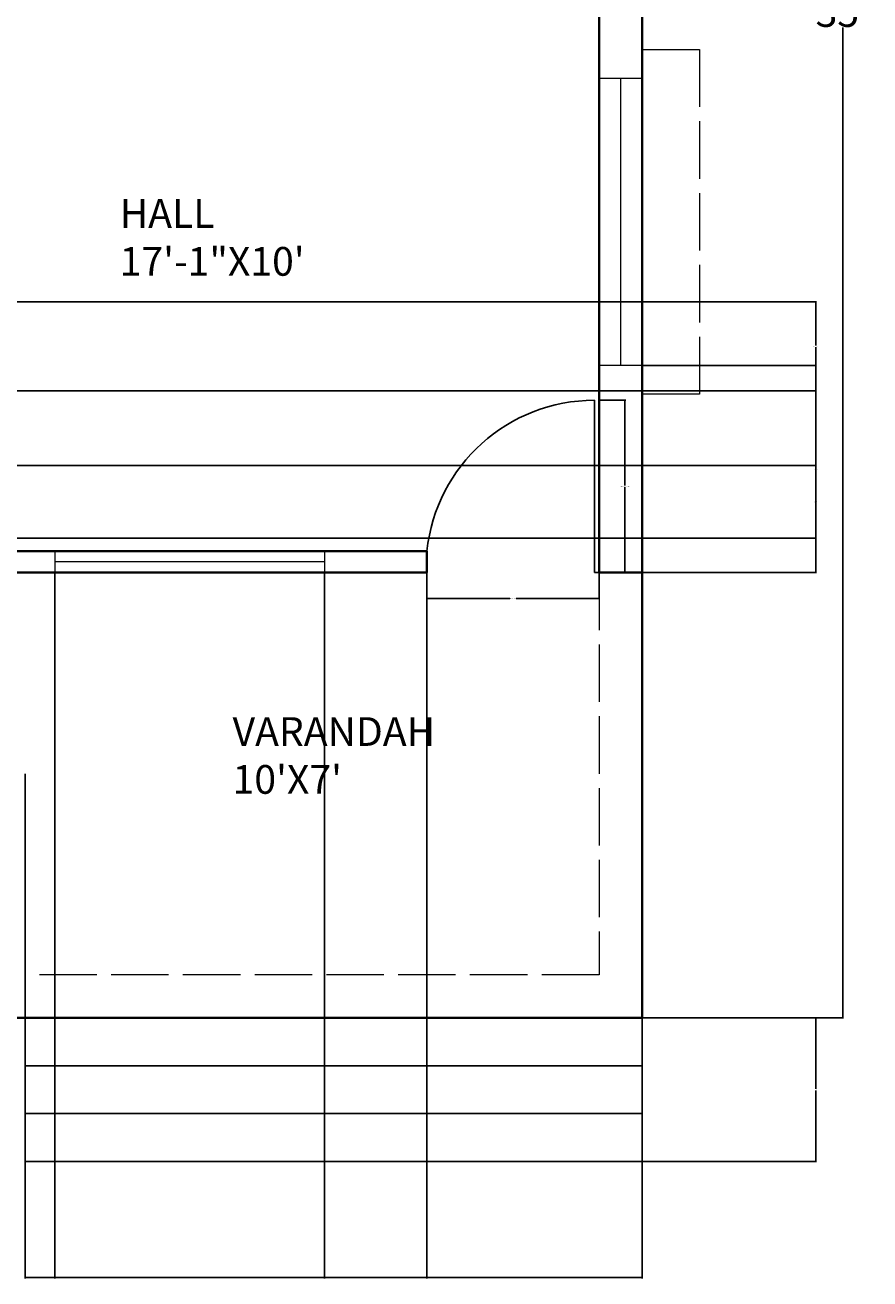
# Model space of a CAD drawing. Units: inches. Extents: x -22 to 362, y -469 to 42.
# Tile 3 of 6: x 186 to 362, y -469 to -207. Entities that reach past the tile are written whole.
import ezdxf

# ---------------------------------------------------------------- set-up
doc = ezdxf.new("R2010")
doc.units = ezdxf.units.IN
doc.header["$MEASUREMENT"] = 0
doc.linetypes.add('ACAD_ISO02W100', pattern=[15, 12, -3])
for name, color, linetype, lineweight in [('A-ANNO-DIMS', 2, 'Continuous', 18), ('A-AREA-IDEN', 7, 'Continuous', 25), ('A-DOOR', 3, 'Continuous', 25), ('A-FLOR-STRS', 7, 'Continuous', 25), ('A-GLAZ', 4, 'Continuous', 20), ('A-ROOF-OVHD', 8, 'ACAD_ISO02W100', 18), ('A-WALL', 7, 'Continuous', 40), ('A-WALL-OVHD', 7, 'ACAD_ISO02W100', 18)]:
    doc.layers.add(name, color=color, linetype=linetype, lineweight=lineweight)
doc.styles.get("Standard").update_dxf_attribs({"font": 'arial.ttf'})
doc.dimstyles.get("Standard").update_dxf_attribs({"dimtxt": 0.18, "dimasz": 0.18, "dimexe": 0.18, "dimexo": 0.0625, "dimgap": 0.09, "dimtad": 0, "dimtih": 1, "dimtoh": 1, "dimdec": 0, "dimzin": 0, "dimdsep": 46, "dimlunit": 3, "dimtxsty": 'Standard', "dimcen": 0.09, "dimadec": 0, "dimazin": 0, "dimtfac": 1, "dimtdec": 0, "dimtofl": 0, "dimtmove": 0, "dimatfit": 3, "dimfxl": 1, "dimtolj": 1, "dimtzin": 0, "dimarcsym": 0})

# ---------------------------------------------------------------- blocks, each defined once
blk = doc.blocks.new('*D6')
at = {"layer": 'A-ANNO-DIMS', "color": 0, "lineweight": -2, "transparency": 16777216}
for p, q in [((314.57, 5.69), (356.62, 5.69)), ((356.44, 5.51), (356.44, -201.15)), ((356.44, -414.13), (356.44, -207.46)), ((314.57, -414.31), (356.62, -414.31))]:
    blk.add_line(p, q, dxfattribs=at)
at = {"layer": 'A-ANNO-DIMS', "color": 0, "transparency": 16777216}
for points in [[(356.41, 5.51), (356.47, 5.51), (356.44, 5.69)], [(356.41, -414.13), (356.47, -414.13), (356.44, -414.31)]]:
    blk.add_solid(points, dxfattribs=at)
at = {"layer": 'Defpoints', "color": 0, "transparency": 16777216}
for p in [(314.51, 5.69), (314.51, -414.31), (356.44, -414.31)]:
    blk.add_point(p, dxfattribs=at)
at = {"layer": 'A-ANNO-DIMS', "color": 0, "transparency": 16777216, "insert": (356.44, -204.31), "char_height": 6, "attachment_point": 5}
blk.add_mtext("\\A1;35'", dxfattribs=at)
blk = doc.blocks.new('DOOR-SWING-36')
for p, q in [((-1, 0), (-1, 36)), ((0, 0), (-1, 0))]:
    blk.add_line(p, q)
blk.add_arc((-1, 0.81), 35.19, 90, 173.9744)
blk = doc.blocks.new('WIN-60-WALL9')
for p, q in [((0, 9), (60, 9)), ((0, 0), (0, 9)), ((60, 9), (60, 0)), ((0, 4.5), (60, 4.5)), ((60, 0), (0, 0))]:
    blk.add_line(p, q)
blk = doc.blocks.new('*D18')
at = {"layer": 'A-ANNO-DIMS', "color": 0, "lineweight": -2, "transparency": 16777216}
for p, q in [((305.57, -285.31), (311.09, -285.31)), ((310.91, -285.49), (310.91, -303.12)), ((310.91, -321.13), (310.91, -303.49)), ((305.57, -321.31), (311.09, -321.31))]:
    blk.add_line(p, q, dxfattribs=at)
at = {"layer": 'A-ANNO-DIMS', "color": 0, "transparency": 16777216}
for points in [[(310.88, -285.49), (310.94, -285.49), (310.91, -285.31)], [(310.88, -321.13), (310.94, -321.13), (310.91, -321.31)]]:
    blk.add_solid(points, dxfattribs=at)
at = {"layer": 'Defpoints', "color": 0, "transparency": 16777216}
for p in [(305.51, -285.31), (310.91, -285.31), (305.51, -321.31)]:
    blk.add_point(p, dxfattribs=at)
at = {"layer": 'A-ANNO-DIMS', "color": 0, "transparency": 16777216, "insert": (310.91, -303.31), "char_height": 0.18, "attachment_point": 5}
blk.add_mtext('\\A1;DOOR 3\'-0" TYP.', dxfattribs=at)
blk = doc.blocks.new('*D19')
at = {"layer": 'A-ANNO-DIMS', "color": 0, "lineweight": -2, "transparency": 16777216}
for p, q in [((269.51, -321.37), (269.51, -326.89)), ((305.51, -321.37), (305.51, -326.89)), ((269.69, -326.71), (286.87, -326.71)), ((305.33, -326.71), (288.15, -326.71))]:
    blk.add_line(p, q, dxfattribs=at)
at = {"layer": 'A-ANNO-DIMS', "color": 0, "transparency": 16777216}
for points in [[(269.69, -326.68), (269.69, -326.74), (269.51, -326.71)], [(305.33, -326.68), (305.33, -326.74), (305.51, -326.71)]]:
    blk.add_solid(points, dxfattribs=at)
at = {"layer": 'Defpoints', "color": 0, "transparency": 16777216}
for p in [(269.51, -321.31), (305.51, -321.31), (305.51, -326.71)]:
    blk.add_point(p, dxfattribs=at)
at = {"layer": 'A-ANNO-DIMS', "color": 0, "transparency": 16777216, "insert": (287.51, -326.71), "char_height": 0.18, "attachment_point": 5}
blk.add_mtext('\\A1;3\'-0" TYP.', dxfattribs=at)
blk = doc.blocks.new('*D41')
at = {"layer": 'A-ANNO-DIMS', "color": 0, "lineweight": -2, "transparency": 16777216}
for p, q in [((314.57, -278.04), (350.97, -278.04)), ((350.79, -278.22), (350.79, -299.49)), ((350.79, -321.13), (350.79, -299.86)), ((314.57, -321.31), (350.97, -321.31))]:
    blk.add_line(p, q, dxfattribs=at)
at = {"layer": 'A-ANNO-DIMS', "color": 0, "transparency": 16777216}
for points in [[(350.76, -278.22), (350.82, -278.22), (350.79, -278.04)], [(350.76, -321.13), (350.82, -321.13), (350.79, -321.31)]]:
    blk.add_solid(points, dxfattribs=at)
at = {"layer": 'Defpoints', "color": 0, "transparency": 16777216}
for p in [(314.51, -278.04), (314.51, -321.31), (350.79, -321.31)]:
    blk.add_point(p, dxfattribs=at)
at = {"layer": 'A-ANNO-DIMS', "color": 0, "transparency": 16777216, "insert": (350.79, -299.68), "char_height": 0.18, "attachment_point": 5}
blk.add_mtext('\\A1;3\'-7 1/2"', dxfattribs=at)
blk = doc.blocks.new('*D42')
at = {"layer": 'A-ANNO-DIMS', "color": 0, "lineweight": -2, "transparency": 16777216}
for p, q in [((185.51, -444.37), (185.51, -468.77)), ((314.51, -444.37), (314.51, -468.77)), ((185.69, -468.59), (249.62, -468.59)), ((314.33, -468.59), (250.4, -468.59))]:
    blk.add_line(p, q, dxfattribs=at)
at = {"layer": 'A-ANNO-DIMS', "color": 0, "transparency": 16777216}
for points in [[(185.69, -468.56), (185.69, -468.62), (185.51, -468.59)], [(314.33, -468.56), (314.33, -468.62), (314.51, -468.59)]]:
    blk.add_solid(points, dxfattribs=at)
at = {"layer": 'Defpoints', "color": 0, "transparency": 16777216}
for p in [(185.51, -444.31), (314.51, -444.31), (314.51, -468.59)]:
    blk.add_point(p, dxfattribs=at)
at = {"layer": 'A-ANNO-DIMS', "color": 0, "transparency": 16777216, "insert": (250.01, -468.59), "char_height": 0.18, "attachment_point": 5}
blk.add_mtext('\\A1;10\'-9"', dxfattribs=at)
blk = doc.blocks.new('*D43')
at = {"layer": 'A-ANNO-DIMS', "color": 0, "lineweight": -2, "transparency": 16777216}
for p, q in [((314.57, -414.31), (350.97, -414.31)), ((350.79, -414.49), (350.79, -429.12)), ((350.79, -444.13), (350.79, -429.49)), ((314.57, -444.31), (350.97, -444.31))]:
    blk.add_line(p, q, dxfattribs=at)
at = {"layer": 'A-ANNO-DIMS', "color": 0, "transparency": 16777216}
for points in [[(350.76, -414.49), (350.82, -414.49), (350.79, -414.31)], [(350.76, -444.13), (350.82, -444.13), (350.79, -444.31)]]:
    blk.add_solid(points, dxfattribs=at)
at = {"layer": 'Defpoints', "color": 0, "transparency": 16777216}
for p in [(314.51, -414.31), (350.79, -414.31), (314.51, -444.31)]:
    blk.add_point(p, dxfattribs=at)
at = {"layer": 'A-ANNO-DIMS', "color": 0, "transparency": 16777216, "insert": (350.79, -429.31), "char_height": 0.18, "attachment_point": 5}
blk.add_mtext('\\A1;2\'-6"', dxfattribs=at)
blk = doc.blocks.new('*D47')
at = {"layer": 'A-ANNO-DIMS', "color": 0, "lineweight": -2, "transparency": 16777216}
for p, q in [((191.73, -321.37), (191.73, -468.77)), ((248.08, -321.37), (248.08, -468.77)), ((191.91, -468.59), (219.36, -468.59)), ((247.9, -468.59), (220.45, -468.59))]:
    blk.add_line(p, q, dxfattribs=at)
at = {"layer": 'A-ANNO-DIMS', "color": 0, "transparency": 16777216}
for points in [[(191.91, -468.56), (191.91, -468.62), (191.73, -468.59)], [(247.9, -468.56), (247.9, -468.62), (248.08, -468.59)]]:
    blk.add_solid(points, dxfattribs=at)
at = {"layer": 'Defpoints', "color": 0, "transparency": 16777216}
for p in [(191.73, -321.31), (248.08, -321.31), (248.08, -468.59)]:
    blk.add_point(p, dxfattribs=at)
at = {"layer": 'A-ANNO-DIMS', "color": 0, "transparency": 16777216, "insert": (219.9, -468.59), "char_height": 0.18, "attachment_point": 5}
blk.add_mtext('\\A1;4\'-8 1/2"', dxfattribs=at)
blk = doc.blocks.new('*D48')
at = {"layer": 'A-ANNO-DIMS', "color": 0, "lineweight": -2, "transparency": 16777216}
for p, q in [((248.08, -321.37), (248.08, -468.77)), ((269.51, -321.37), (269.51, -468.77)), ((248.26, -468.59), (258.26, -468.59)), ((269.33, -468.59), (259.32, -468.59))]:
    blk.add_line(p, q, dxfattribs=at)
at = {"layer": 'A-ANNO-DIMS', "color": 0, "transparency": 16777216}
for points in [[(248.26, -468.56), (248.26, -468.62), (248.08, -468.59)], [(269.33, -468.56), (269.33, -468.62), (269.51, -468.59)]]:
    blk.add_solid(points, dxfattribs=at)
at = {"layer": 'Defpoints', "color": 0, "transparency": 16777216}
for p in [(248.08, -321.31), (269.51, -321.31), (269.51, -468.59)]:
    blk.add_point(p, dxfattribs=at)
at = {"layer": 'A-ANNO-DIMS', "color": 0, "transparency": 16777216, "insert": (258.79, -468.59), "char_height": 0.18, "attachment_point": 5}
blk.add_mtext('\\A1;1\'-9 1/2"', dxfattribs=at)
blk = doc.blocks.new('*D57')
at = {"layer": 'A-ANNO-DIMS', "color": 0, "lineweight": -2, "transparency": 16777216}
for p, q in [((146.47, -264.76), (350.97, -264.76)), ((350.79, -264.94), (350.79, -273.87)), ((350.79, -283.16), (350.79, -274.23)), ((146.47, -283.34), (350.97, -283.34))]:
    blk.add_line(p, q, dxfattribs=at)
at = {"layer": 'A-ANNO-DIMS', "color": 0, "transparency": 16777216}
for points in [[(350.76, -264.94), (350.82, -264.94), (350.79, -264.76)], [(350.76, -283.16), (350.82, -283.16), (350.79, -283.34)]]:
    blk.add_solid(points, dxfattribs=at)
at = {"layer": 'Defpoints', "color": 0, "transparency": 16777216}
for p in [(146.41, -264.76), (146.41, -283.34), (350.79, -283.34)]:
    blk.add_point(p, dxfattribs=at)
at = {"layer": 'A-ANNO-DIMS', "color": 0, "transparency": 16777216, "insert": (350.79, -274.05), "char_height": 0.18, "attachment_point": 5}
blk.add_mtext('\\A1;1\'-6 1/2"', dxfattribs=at)
blk = doc.blocks.new('*D61')
at = {"layer": 'A-ANNO-DIMS', "color": 0, "lineweight": -2, "transparency": 16777216}
for p, q in [((92.28, -298.96), (350.97, -298.96)), ((350.79, -299.14), (350.79, -306.36)), ((350.79, -313.95), (350.79, -306.73)), ((93.96, -314.13), (350.97, -314.13))]:
    blk.add_line(p, q, dxfattribs=at)
at = {"layer": 'A-ANNO-DIMS', "color": 0, "transparency": 16777216}
for points in [[(350.76, -299.14), (350.82, -299.14), (350.79, -298.96)], [(350.76, -313.95), (350.82, -313.95), (350.79, -314.13)]]:
    blk.add_solid(points, dxfattribs=at)
at = {"layer": 'Defpoints', "color": 0, "transparency": 16777216}
for p in [(92.21, -298.96), (350.79, -298.96), (93.9, -314.13)]:
    blk.add_point(p, dxfattribs=at)
at = {"layer": 'A-ANNO-DIMS', "color": 0, "transparency": 16777216, "insert": (350.79, -306.55), "char_height": 0.18, "attachment_point": 5}
blk.add_mtext('\\A1;1\'-3"', dxfattribs=at)

msp = doc.modelspace()

# ---------------------------------------------------------------- linework, layer by layer
at = {"layer": 'A-FLOR-STRS'}
for p, q in [((185.51, -363.31), (185.51, -405.31)), ((185.51, -405.31), (185.51, -414.31)), ((185.51, -414.31), (185.51, -424.31)), ((314.51, -444.31), (314.51, -414.31)), ((185.51, -424.31), (185.51, -434.31)), ((185.51, -424.31), (314.51, -424.31)), ((185.51, -434.31), (185.51, -444.31)), ((185.51, -434.31), (314.51, -434.31)), ((185.51, -444.31), (314.51, -444.31))]:
    msp.add_line(p, q, dxfattribs=at)
at = {"layer": 'A-GLAZ'}
for p, q in [((191.73, -316.81), (191.73, -321.31)), ((248.08, -316.81), (248.08, -321.31)), ((248.08, -319.06), (191.73, -319.06))]:
    msp.add_line(p, q, dxfattribs=at)
at = {"layer": 'A-ROOF-OVHD'}
for p, q in [((314.51, -212.04), (326.51, -212.04)), ((326.51, -212.04), (326.51, -278.04)), ((326.51, -278.04), (326.51, -284.04)), ((326.51, -284.04), (314.51, -284.04))]:
    msp.add_line(p, q, dxfattribs=at)
at = {"layer": 'A-WALL'}
for p, q in [((314.51, 5.69), (314.51, -414.31)), ((305.51, -196.81), (305.51, -321.31)), ((100.51, -316.81), (269.51, -316.81)), ((269.51, -316.81), (269.51, -321.31)), ((24.01, -321.31), (269.51, -321.31)), ((305.51, -321.31), (314.51, -321.31)), ((15.01, -414.31), (314.51, -414.31))]:
    msp.add_line(p, q, dxfattribs=at)
at = {"layer": 'A-WALL-OVHD'}
for p, q in [((305.51, -321.31), (305.51, -405.31)), ((305.51, -405.31), (185.51, -405.31))]:
    msp.add_line(p, q, dxfattribs=at)

# ---------------------------------------------------------------- block references
at = {"layer": 'A-DOOR'}
msp.add_blockref('DOOR-SWING-36', (305.51, -321.31), dxfattribs=at)
at = {"layer": 'A-GLAZ', "rotation": 270}
msp.add_blockref('WIN-60-WALL9', (305.51, -218.04), dxfattribs=at)

# ---------------------------------------------------------------- texts
at = {"layer": 'A-AREA-IDEN', "char_height": 6, "attachment_point": 1}
for s, insert in [('HALL\\P17\'-1"X10\'', (205.29, -243.29)), ("VARANDAH\\P10'X7'", (228.89, -351.51))]:
    msp.add_mtext(s, dxfattribs=dict(at, insert=insert))

# ---------------------------------------------------------------- dimensions: what is measured, and where the dimension line sits
at = {"layer": 'A-ANNO-DIMS'}
for base, p1, p2, override, picture, middle in [((356.44, -414.31), (314.51, 5.69), (314.51, -414.31), {"dimtxt": 6, "dimclrd": 0, "dimclre": 0, "dimclrt": 0}, '*D6', (356.44, -204.31)), ((350.79, -283.34), (146.41, -264.76), (146.41, -283.34), {"dimdec": 1, "dimlfac": 1, "dimrnd": 0, "dimzin": 1, "dimdsep": 46, "dimlunit": 4, "dimfrac": 2}, '*D57', (350.79, -274.05)), ((350.79, -321.31), (314.51, -278.04), (314.51, -321.31), {"dimdec": 1, "dimlfac": 1, "dimrnd": 0, "dimzin": 1, "dimdsep": 46, "dimlunit": 4, "dimfrac": 2}, '*D41', (350.79, -299.68)), ((350.79, -298.96), (93.9, -314.13), (92.21, -298.96), {"dimdec": 1, "dimlfac": 1, "dimrnd": 0, "dimzin": 1, "dimdsep": 46, "dimlunit": 4, "dimfrac": 2}, '*D61', (350.79, -306.55)), ((350.79, -414.31), (314.51, -444.31), (314.51, -414.31), {"dimdec": 1, "dimlfac": 1, "dimrnd": 0, "dimzin": 1, "dimdsep": 46, "dimlunit": 4, "dimfrac": 2}, '*D43', (350.79, -429.31))]:
    dim = msp.add_linear_dim(base=base, p1=p1, p2=p2, angle=90, dimstyle='Standard', override=override, dxfattribs=at)
    dim.commit()
    dim.dimension.update_dxf_attribs({"geometry": picture, "text_midpoint": middle})
dim = msp.add_linear_dim(base=(310.91, -285.31), p1=(305.51, -321.31), p2=(305.51, -285.31), angle=90, text='DOOR <> TYP.', dimstyle='Standard', override={"dimdec": 1, "dimlfac": 1, "dimrnd": 0, "dimzin": 1, "dimdsep": 46, "dimlunit": 4, "dimfrac": 2}, dxfattribs=at)
dim.commit()
dim.dimension.update_dxf_attribs({"geometry": '*D18', "text_midpoint": (310.91, -303.31)})
for base, p1, p2, picture, middle in [((248.07754, -468.58659), (191.72752, -321.30659), (248.07754, -321.30659), '*D47', (219.90253, -468.58659)), ((269.51, -468.59), (248.08, -321.31), (269.51, -321.31), '*D48', (258.79, -468.59)), ((314.51, -468.59), (185.51, -444.31), (314.51, -444.31), '*D42', (250.01, -468.59))]:
    dim = msp.add_linear_dim(base=base, p1=p1, p2=p2, dimstyle='Standard', override={"dimdec": 1, "dimlfac": 1, "dimrnd": 0, "dimzin": 1, "dimdsep": 46, "dimlunit": 4, "dimfrac": 2}, dxfattribs=at)
    dim.commit()
    dim.dimension.update_dxf_attribs({"geometry": picture, "text_midpoint": middle})
dim = msp.add_linear_dim(base=(305.51, -326.71), p1=(269.51, -321.31), p2=(305.51, -321.31), text='<> TYP.', dimstyle='Standard', override={"dimdec": 1, "dimlfac": 1, "dimrnd": 0, "dimzin": 1, "dimdsep": 46, "dimlunit": 4, "dimfrac": 2}, dxfattribs=at)
dim.commit()
dim.dimension.update_dxf_attribs({"geometry": '*D19', "text_midpoint": (287.51, -326.71)})

doc.saveas('drawing.dxf')
